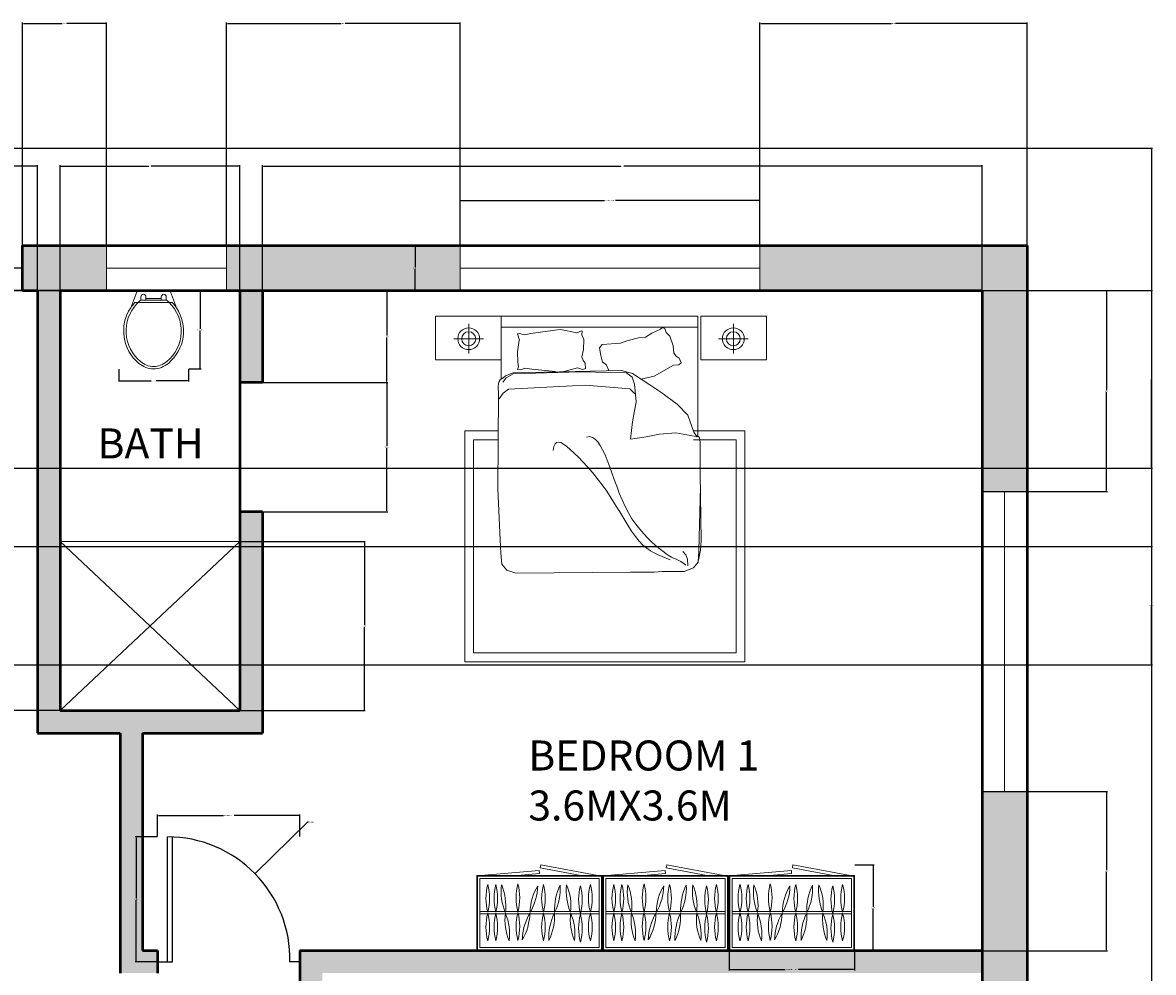
# Model space of a CAD drawing. Units: inches. Extents: x 3 to 380, y -485 to 60.
# Tile 8 of 8: x 154 to 380, y -130 to 60. Entities that reach past the tile are written whole.
import ezdxf

# ---------------------------------------------------------------- set-up
doc = ezdxf.new("R2010")
doc.units = ezdxf.units.IN
doc.header["$MEASUREMENT"] = 0
for name, color, linetype, lineweight in [('A-ANNO-DIMS', 2, 'Continuous', 18), ('A-AREA-IDEN', 7, 'Continuous', 25), ('A-DOOR', 3, 'Continuous', 25), ('A-FLOR-FIXT', 9, 'Continuous', 18), ('A-FURN', 8, 'Continuous', 18), ('A-GLAZ', 4, 'Continuous', 18), ('A-WALL', 7, 'Continuous', 50), ('A-WALL-PATT', 252, 'Continuous', 13)]:
    doc.layers.add(name, color=color, linetype=linetype, lineweight=lineweight)
doc.styles.get("Standard").update_dxf_attribs({"font": 'arial.ttf'})
doc.dimstyles.get("Standard").update_dxf_attribs({"dimtxt": 0.18, "dimasz": 0.18, "dimexe": 0.18, "dimexo": 0.0625, "dimgap": 0.09, "dimtad": 0, "dimtih": 1, "dimtoh": 1, "dimdec": 0, "dimzin": 0, "dimdsep": 46, "dimlunit": 3, "dimtxsty": 'Standard', "dimcen": 0.09, "dimadec": 0, "dimazin": 0, "dimtfac": 1, "dimtdec": 0, "dimtofl": 0, "dimtmove": 0, "dimatfit": 3, "dimfxl": 1, "dimtolj": 1, "dimtzin": 0, "dimarcsym": 0})

# ---------------------------------------------------------------- blocks, each defined once
blk = doc.blocks.new('BED-DOUBLE-WITH-NIGHTSTANDS')
for p, q in [((13.15, 56.48), (13.15, 69.11)), ((6.62, 67.56), (6.62, 61.62)), ((25.02, 66.47), (23.83, 66.33)), ((28.24, 65.8), (25.02, 66.47)), ((29.23, 66.16), (28.24, 65.8)), ((29.33, 66.13), (29.23, 66.16)), ((29.33, 66.13), (29.25, 65.4)), ((29.33, 66.13), (29.25, 65.4)), ((42.02, 64.91), (43.24, 65.73)), ((42.02, 64.91), (43.24, 65.73)), ((43.24, 65.73), (44.98, 66.53)), ((46.15, 65.85), (46.84, 65.09)), ((59.58, 67.56), (59.58, 61.62)), ((3.65, 64.59), (9.59, 64.59)), ((16.76, 64.3), (16.42, 65.57)), ((29.25, 65.4), (29.65, 64.45)), ((29.65, 64.45), (29.63, 62.44)), ((33.33, 63.47), (37.02, 63.69)), ((37.02, 63.69), (38.27, 64.16)), ((38.27, 64.16), (40.63, 64.79)), ((40.63, 64.79), (42.02, 64.91)), ((46.84, 65.09), (47.51, 63.2)), ((62.55, 64.59), (56.61, 64.59)), ((29.63, 62.44), (29.27, 60.96)), ((47.51, 63.2), (47.67, 61.68)), ((47.67, 61.68), (48.15, 61.09)), ((29.27, 60.96), (29.52, 60.24)), ((29.52, 60.24), (29.96, 59.68)), ((29.96, 59.68), (30.03, 58.63)), ((47.6, 59.3), (43.73, 57.13)), ((48.66, 59.34), (47.6, 59.3)), ((48.15, 61.09), (48.75, 60.71)), ((49.17, 59.74), (48.66, 59.34)), ((48.75, 60.71), (49.17, 59.74)), ((28.4, 58.75), (25.21, 57.93)), ((29.41, 58.43), (28.4, 58.75)), ((30.03, 58.63), (29.41, 58.43)), ((12.59, 55.61), (12.54, 55)), ((12.54, 55), (12.56, 53.58)), ((12.56, 53.58), (12.48, 34.55)), ((52.39, 45), (52.46, 45.03)), ((52.97, 37.68), (52.91, 43.85)), ((53.11, 24.16), (52.97, 37.68)), ((12.48, 34.55), (12.89, 24.35)), ((53.02, 35.03), (52.75, 24.82)), ((12.89, 24.35), (13.03, 21.68)), ((52.75, 24.82), (52.69, 22.14)), ((53, 22.29), (53.11, 24.16)), ((13.03, 21.68), (13.27, 19.48)), ((50.1, 21.39), (49.46, 22.06)), ((50.39, 20.5), (50.1, 21.39)), ((50.45, 19.2), (50.39, 20.5)), ((52.69, 22.14), (52.52, 19.94)), ((52.63, 20.34), (53, 22.29)), ((13.27, 19.48), (14.23, 18.32)), ((14.23, 18.32), (16.09, 17.69)), ((51.59, 18.75), (49.75, 18.06)), ((52.52, 19.94), (51.59, 18.75)), ((39.03, 17.94), (16.09, 17.69)), ((39.03, 17.94), (43.71, 17.94)), ((43.71, 17.94), (45.37, 18.06)), ((45.37, 18.06), (49.75, 18.06))]:
    blk.add_line(p, q)
for points in [[(0, 60.38), (13.1, 60.38), (13.1, 69.11), (0, 69.11)], [(66.2, 60.38), (53.1, 60.38), (53.1, 69.11), (66.2, 69.11)]]:
    blk.add_lwpolyline(points, close=True)
for points in [[(13.15, 69.11), (52.45, 69.11), (52.45, 45.06)], [(52.45, 66.93), (13.15, 66.93)], [(23.83, 66.33), (19.08, 65.62), (17.7, 65.39), (16.88, 65.65), (16.42, 65.57)], [(46.15, 65.85), (45.9, 66.66), (45.38, 66.82), (44.98, 66.53)], [(24.02, 58.01), (19.24, 58.51), (17.85, 58.68), (17.04, 58.38), (16.37, 58.47), (16.56, 59), (16.45, 59.9), (16.42, 62), (16.71, 64.3)], [(33.33, 63.47), (32.82, 62.74), (33.06, 61.23), (33.43, 59.89), (34.16, 59.47), (34.58, 58.37), (34.59, 58.17)], [(12.61, 55.65), (12.74, 56.06), (12.92, 56.37), (13.15, 56.48), (13.4, 56.7), (13.44, 56.72)], [(52.45, 44.97), (48.05, 45.75), (44.8, 45.5), (42.14, 44.97), (38.99, 44.52), (39.41, 47.96), (40.12, 51.96), (39.81, 55.5), (39.35, 56.93), (38.2, 57.74), (28.88, 58), (15.49, 57.6), (14.12, 56.79), (13.54, 55.99), (13.47, 55.91)], [(13.48, 56.71), (14.02, 57.18), (15.49, 57.8), (37.2, 58.22), (39.38, 57.66), (42.87, 55.35), (45.06, 53.9), (48.36, 51.48), (50.46, 49.34), (51.7, 45.9), (52.31, 45)], [(43.73, 57.13), (41.15, 56.49)], [(39.86, 53.54), (38.87, 54.55), (30.01, 55.3), (27.42, 55.15), (14.59, 54.51), (13.51, 53.69), (12.69, 52.6)], [(51.61, 46.15), (61.88, 46.15), (61.88, 0), (5.85, 0), (5.85, 46.15), (12.53, 46.15)], [(51.61, 44.4), (60.14, 44.4), (60.14, 1.75), (7.59, 1.75), (7.59, 44.4), (12.53, 44.4)], [(46.96, 20.37), (46.12, 20.73), (45.31, 21.07), (44.52, 21.41), (43.75, 21.77), (42.99, 22.2), (42.24, 22.71), (41.49, 23.33), (40.74, 24.1), (39.99, 25.04), (39.23, 26.12), (38.46, 27.32), (37.67, 28.61), (36.87, 29.96), (36.03, 31.34), (35.16, 32.73), (34.26, 34.09), (33.32, 35.4), (32.36, 36.66), (31.39, 37.84), (30.42, 38.95), (29.48, 39.98), (28.57, 40.91), (27.72, 41.73), (26.93, 42.45), (26.23, 43.05), (25.61, 43.51), (25.06, 43.81), (24.6, 43.93), (24.22, 43.85), (23.91, 43.56), (23.68, 43.04), (23.52, 42.25)], [(50.06, 19.34), (49.7, 19.62), (49.37, 19.84), (49.06, 20.03), (48.78, 20.19), (48.52, 20.33), (48.27, 20.44), (48.02, 20.55), (47.76, 20.67), (47.5, 20.79), (47.21, 20.93), (46.9, 21.1), (46.56, 21.31), (46.16, 21.57), (45.71, 21.89), (45.2, 22.29), (44.61, 22.76), (43.95, 23.32), (43.23, 23.98), (42.45, 24.72), (41.66, 25.56), (40.85, 26.48), (40.05, 27.49), (39.29, 28.58), (38.57, 29.76), (37.91, 31.03), (37.31, 32.35), (36.75, 33.71), (36.24, 35.08), (35.75, 36.45), (35.28, 37.79), (34.82, 39.08), (34.36, 40.29), (33.9, 41.4), (33.43, 42.39), (32.94, 43.25), (32.44, 43.96), (31.91, 44.5), (31.37, 44.86), (30.8, 45.01), (30.2, 44.94)], [(52.91, 43.91), (52.84, 44.76), (52.6, 45.01), (52.45, 45.06)]]:
    blk.add_lwpolyline(points)
for centre, radius in [((6.62, 64.59), 2.18), ((6.62, 64.59), 1.4), ((59.58, 64.59), 2.18), ((59.58, 64.59), 1.4)]:
    blk.add_circle(centre, radius)
blk = doc.blocks.new('WC-PLAN')
for p, q in [((2.25, 13.31), (2.91, 13.31)), ((2.91, 13.31), (5.99, 13.31)), ((9.08, 13.31), (5.99, 13.31)), ((9.08, 13.31), (9.73, 13.31))]:
    blk.add_line(p, q)
for points in [[(5.99, 15.68), (3, 15.68, 0.31031), (2.63, 15.43), (1.4, 12.23, 0.209071)], [(3.45, 13.78, 0.022712), (2.91, 13.31, 0.162618)], [(3.45, 13.78), (3.45, 14.44, -1), (4.45, 14.44), (4.45, 14.1)], [(5.99, 13.78), (3.45, 13.78, 0.022712)], [(5.99, 15.68), (8.98, 15.68, -0.31031), (9.35, 15.43), (10.58, 12.23, -0.209071)], [(5.99, 13.78), (8.53, 13.78, -0.476108)], [(8.53, 13.78), (8.53, 14.44, 1), (7.53, 14.44), (7.53, 14.1)], [(8.53, 13.78, -0.022712), (9.08, 13.31, -0.162618)], [(1.4, 12.23, 0.383919), (3.04, 1.13, 0.163732), (5.99, 0, 0.359733)], [(2.59, 12.99, 0.431639), (3.34, 1.49, 0.162618), (5.99, 0.47, 0.470877)], [(2.25, 13.31, 0.040937), (1.4, 12.23, 0.163732)], [(2.91, 13.31, 0.014165), (2.59, 12.99, 0.162618)], [(9.08, 13.31, -0.448546), (8.64, 1.49, -0.162618), (5.99, 0.47, -0.470877)], [(10.58, 12.23, -0.383919), (8.94, 1.13, -0.163732), (5.99, 0, -0.359733)], [(9.73, 13.31, -0.040937), (10.58, 12.23, -0.163732)]]:
    blk.add_lwpolyline(points, format="xyb")
for points in [[(7.53, 14.1), (4.45, 14.1)], [(4.45, 14.1), (4.45, 13.78)], [(7.53, 14.1), (7.53, 13.78)]]:
    blk.add_lwpolyline(points)
blk = doc.blocks.new('WARDROBE-MODULE')
for p, q in [((0.61, 7.83), (24.49, 7.83)), ((0.61, 7.39), (24.49, 7.39))]:
    blk.add_line(p, q)
for points in [[(0.79, 15.06), (12.48, 16.03), (12.53, 15.42), (8.15, 15.06)], [(24.21, 15.06), (12.8, 17.14), (12.69, 16.54), (20.81, 15.06)]]:
    blk.add_lwpolyline(points)
for points in [[(0, 0), (25.1, 0), (25.1, 15.06), (0, 15.06)], [(0.14, 0.14), (24.96, 0.14), (24.96, 14.92), (0.14, 14.92)], [(0.61, 0.61), (24.49, 0.61), (24.49, 14.45), (0.61, 14.45)]]:
    blk.add_lwpolyline(points, close=True)
for centre, start, end in [((12.71, 10.45), 165.1905, 194.8095), ((-8.32, 10.45), 345.1905, 14.8095), ((14.34, 10.45), 165.1905, 194.8095), ((-6.7, 10.45), 345.1905, 14.8095), ((15.77, 11.77), 172.7904, 202.4093), ((-5.07, 8.99), 352.7904, 22.4093), ((18.76, 10.57), 165.1905, 194.8095), ((-2.27, 10.57), 345.1905, 14.8095), ((1.32, 13.21), 329.2346, 358.8535), ((21.55, 7.43), 149.2346, 178.8535), ((23.87, 10.45), 165.1905, 194.8095), ((2.84, 10.45), 345.1905, 14.8095), ((26.45, 8.28), 153.6481, 183.267), ((5.84, 12.49), 333.6481, 3.267), ((28.79, 11.91), 173.3262, 202.9452), ((7.97, 8.93), 353.3262, 22.9452), ((31.27, 10.2), 165.1905, 194.8095), ((10.24, 10.2), 345.1905, 14.8095), ((33.25, 10.45), 165.1905, 194.8095), ((12.22, 10.45), 345.1905, 14.8095), ((12.71, 4.73), 165.1905, 194.8095), ((-8.32, 4.73), 345.1905, 14.8095), ((14.34, 4.73), 165.1905, 194.8095), ((-6.7, 4.73), 345.1905, 14.8095), ((16.53, 6.1), 172.7904, 202.4093), ((-4.32, 3.32), 352.7904, 22.4093), ((18.76, 4.84), 165.1905, 194.8095), ((-2.27, 4.84), 345.1905, 14.8095), ((19.98, 1.92), 149.2346, 178.8535), ((-0.25, 7.71), 329.2346, 358.8535), ((23.87, 4.73), 165.1905, 194.8095), ((2.84, 4.73), 345.1905, 14.8095), ((25.3, 2.68), 153.6481, 183.267), ((4.69, 6.89), 333.6481, 3.267), ((29.6, 6.25), 173.3262, 202.9452), ((8.78, 3.27), 353.3262, 22.9452), ((31.27, 4.48), 165.1905, 194.8095), ((10.24, 4.48), 345.1905, 14.8095), ((33.25, 4.73), 165.1905, 194.8095), ((12.22, 4.73), 345.1905, 14.8095)]:
    blk.add_arc(centre, 10.88, start, end)
blk = doc.blocks.new('WIN-60X9')
for p, q in [((60, 9), (0, 9)), ((0, 9), (0, 0)), ((60, 0), (60, 9)), ((0, 4.5), (60, 4.5)), ((0, 0), (60, 0))]:
    blk.add_line(p, q)
blk = doc.blocks.new('WIN-24X9')
for p, q in [((0, 24), (0, 0)), ((9, 24), (0, 24)), ((4.5, 24), (4.5, 0)), ((9, 0), (9, 24)), ((0, 0), (9, 0))]:
    blk.add_line(p, q)
blk = doc.blocks.new('DOOR-SWING-24')
for p, q in [((25, 0), (25, 24)), ((26, 0), (26, 24)), ((2, 0), (0, 0)), ((25, 0), (26, 0)), ((28, 0), (26, 0))]:
    blk.add_line(p, q)
blk.add_arc((26, 0), 24, 90, 180)
blk = doc.blocks.new('DOOR-SWING-25')
for p, q in [((2, 0), (2, 25)), ((3, 0), (3, 25)), ((0, 0), (2, 0)), ((2, 0), (3, 0)), ((28.5, 0), (26.5, 0))]:
    blk.add_line(p, q)
blk.add_arc((2, 0.5), 24.5, 358.8425, 90)
blk = doc.blocks.new('*D17')
at = {"layer": 'A-ANNO-DIMS', "color": 0, "lineweight": -2, "transparency": 16777216}
for p, q in [((241.37, 15.23), (241.37, 24.34)), ((241.55, 24.16), (270.26, 24.16)), ((301.19, 24.16), (272.49, 24.16)), ((301.37, 15.23), (301.37, 24.34))]:
    blk.add_line(p, q, dxfattribs=at)
at = {"layer": 'A-ANNO-DIMS', "color": 0, "transparency": 16777216}
for points in [[(241.55, 24.19), (241.55, 24.13), (241.37, 24.16)], [(301.19, 24.19), (301.19, 24.13), (301.37, 24.16)]]:
    blk.add_solid(points, dxfattribs=at)
at = {"layer": 'Defpoints', "color": 0, "transparency": 16777216}
for p in [(301.37, 24.16), (241.37, 15.16), (301.37, 15.16)]:
    blk.add_point(p, dxfattribs=at)
at = {"layer": 'A-ANNO-DIMS', "color": 0, "transparency": 16777216, "insert": (271.37, 24.16), "char_height": 0.18, "attachment_point": 5}
blk.add_mtext('\\A1;WINDOW 60 TYP.', dxfattribs=at)
blk = doc.blocks.new('*D18')
at = {"layer": 'A-ANNO-DIMS', "color": 0, "lineweight": -2, "transparency": 16777216}
for p, q in [((241.31, 15.16), (232.19, 15.16)), ((232.37, 14.98), (232.37, 10.85)), ((232.37, 6.34), (232.37, 10.48)), ((241.31, 6.16), (232.19, 6.16))]:
    blk.add_line(p, q, dxfattribs=at)
at = {"layer": 'A-ANNO-DIMS', "color": 0, "transparency": 16777216}
for points in [[(232.34, 14.98), (232.4, 14.98), (232.37, 15.16)], [(232.34, 6.34), (232.4, 6.34), (232.37, 6.16)]]:
    blk.add_solid(points, dxfattribs=at)
at = {"layer": 'Defpoints', "color": 0, "transparency": 16777216}
for p in [(232.37, 15.16), (241.37, 15.16), (241.37, 6.16)]:
    blk.add_point(p, dxfattribs=at)
at = {"layer": 'A-ANNO-DIMS', "color": 0, "transparency": 16777216, "insert": (232.37, 10.66), "char_height": 0.18, "attachment_point": 5}
blk.add_mtext('\\A1;9 TYP.', dxfattribs=at)
blk = doc.blocks.new('*D25')
at = {"layer": 'A-ANNO-DIMS', "color": 0, "lineweight": -2, "transparency": 16777216}
for p, q in [((180.84, -103.02), (180.84, -98.63)), ((181.02, -98.81), (194.04, -98.81)), ((209.16, -98.81), (196.14, -98.81)), ((209.34, -103.02), (209.34, -98.63))]:
    blk.add_line(p, q, dxfattribs=at)
at = {"layer": 'A-ANNO-DIMS', "color": 0, "transparency": 16777216}
for points in [[(181.02, -98.78), (181.02, -98.84), (180.84, -98.81)], [(209.16, -98.78), (209.16, -98.84), (209.34, -98.81)]]:
    blk.add_solid(points, dxfattribs=at)
at = {"layer": 'Defpoints', "color": 0, "transparency": 16777216}
for p in [(209.34, -98.81), (180.84, -103.09), (209.34, -103.09)]:
    blk.add_point(p, dxfattribs=at)
at = {"layer": 'A-ANNO-DIMS', "color": 0, "transparency": 16777216, "insert": (195.09, -98.81), "char_height": 0.18, "attachment_point": 5}
blk.add_mtext('\\A1;DOOR B 29 TYP.', dxfattribs=at)
blk = doc.blocks.new('*D26')
at = {"layer": 'A-ANNO-DIMS', "color": 0, "lineweight": -2, "transparency": 16777216}
for p, q in [((180.78, -103.09), (176.39, -103.09)), ((176.57, -103.27), (176.57, -115.4)), ((176.57, -127.91), (176.57, -115.77)), ((180.78, -128.09), (176.39, -128.09))]:
    blk.add_line(p, q, dxfattribs=at)
at = {"layer": 'A-ANNO-DIMS', "color": 0, "transparency": 16777216}
for points in [[(176.54, -103.27), (176.6, -103.27), (176.57, -103.09)], [(176.54, -127.91), (176.6, -127.91), (176.57, -128.09)]]:
    blk.add_solid(points, dxfattribs=at)
at = {"layer": 'Defpoints', "color": 0, "transparency": 16777216}
for p in [(176.57, -103.09), (180.84, -103.09), (180.84, -128.09)]:
    blk.add_point(p, dxfattribs=at)
at = {"layer": 'A-ANNO-DIMS', "color": 0, "transparency": 16777216, "insert": (176.57, -115.59), "char_height": 0.18, "attachment_point": 5}
blk.add_mtext('\\A1;25 TYP.', dxfattribs=at)
blk = doc.blocks.new('*D29')
at = {"layer": 'A-ANNO-DIMS', "color": 0, "lineweight": -2, "transparency": 16777216}
for p, q in [((295.2, -125.9), (295.2, -129.78)), ((320.3, -125.9), (320.3, -129.78)), ((295.38, -129.6), (306.44, -129.6)), ((320.12, -129.6), (309.06, -129.6))]:
    blk.add_line(p, q, dxfattribs=at)
at = {"layer": 'A-ANNO-DIMS', "color": 0, "transparency": 16777216}
for points in [[(295.38, -129.57), (295.38, -129.63), (295.2, -129.6)], [(320.12, -129.57), (320.12, -129.63), (320.3, -129.6)]]:
    blk.add_solid(points, dxfattribs=at)
at = {"layer": 'Defpoints', "color": 0, "transparency": 16777216}
for p in [(295.2, -125.84), (320.3, -125.84), (320.3, -129.6)]:
    blk.add_point(p, dxfattribs=at)
at = {"layer": 'A-ANNO-DIMS', "color": 0, "transparency": 16777216, "insert": (307.75, -129.6), "char_height": 0.18, "attachment_point": 5}
blk.add_mtext('\\A1;WARDROBE 25 TYP.', dxfattribs=at)
blk = doc.blocks.new('*D30')
at = {"layer": 'A-ANNO-DIMS', "color": 0, "lineweight": -2, "transparency": 16777216}
for p, q in [((320.36, -108.7), (324.24, -108.7)), ((324.06, -108.88), (324.06, -117.09)), ((324.06, -125.66), (324.06, -117.45)), ((320.36, -125.84), (324.24, -125.84))]:
    blk.add_line(p, q, dxfattribs=at)
at = {"layer": 'A-ANNO-DIMS', "color": 0, "transparency": 16777216}
for points in [[(324.03, -108.88), (324.09, -108.88), (324.06, -108.7)], [(324.03, -125.66), (324.09, -125.66), (324.06, -125.84)]]:
    blk.add_solid(points, dxfattribs=at)
at = {"layer": 'Defpoints', "color": 0, "transparency": 16777216}
for p in [(320.3, -108.7), (324.06, -108.7), (320.3, -125.84)]:
    blk.add_point(p, dxfattribs=at)
at = {"layer": 'A-ANNO-DIMS', "color": 0, "transparency": 16777216, "insert": (324.06, -117.27), "char_height": 0.18, "attachment_point": 5}
blk.add_mtext('\\A1;17 TYP.', dxfattribs=at)
blk = doc.blocks.new('*D33')
at = {"layer": 'A-ANNO-DIMS', "color": 0, "lineweight": -2, "transparency": 16777216}
for p, q in [((187.08, 6.16), (189.55, 6.16)), ((189.37, 5.98), (189.37, -1.49)), ((189.37, -9.34), (189.37, -1.86)), ((187.08, -9.52), (189.55, -9.52))]:
    blk.add_line(p, q, dxfattribs=at)
at = {"layer": 'A-ANNO-DIMS', "color": 0, "transparency": 16777216}
for points in [[(189.34, 5.98), (189.4, 5.98), (189.37, 6.16)], [(189.34, -9.34), (189.4, -9.34), (189.37, -9.52)]]:
    blk.add_solid(points, dxfattribs=at)
at = {"layer": 'Defpoints', "color": 0, "transparency": 16777216}
for p in [(187.02, 6.16), (189.37, 6.16), (187.02, -9.52)]:
    blk.add_point(p, dxfattribs=at)
at = {"layer": 'A-ANNO-DIMS', "color": 0, "transparency": 16777216, "insert": (189.37, -1.68), "char_height": 0.18, "attachment_point": 5}
blk.add_mtext('\\A1;WC 16 TYP.', dxfattribs=at)
blk = doc.blocks.new('*D34')
at = {"layer": 'A-ANNO-DIMS', "color": 0, "lineweight": -2, "transparency": 16777216}
for p, q in [((173.09, -9.58), (173.09, -12.05)), ((187.02, -9.58), (187.02, -12.05)), ((173.27, -11.87), (179.54, -11.87)), ((186.84, -11.87), (180.58, -11.87))]:
    blk.add_line(p, q, dxfattribs=at)
at = {"layer": 'A-ANNO-DIMS', "color": 0, "transparency": 16777216}
for points in [[(173.27, -11.84), (173.27, -11.9), (173.09, -11.87)], [(186.84, -11.84), (186.84, -11.9), (187.02, -11.87)]]:
    blk.add_solid(points, dxfattribs=at)
at = {"layer": 'Defpoints', "color": 0, "transparency": 16777216}
for p in [(173.09, -9.52), (187.02, -9.52), (187.02, -11.87)]:
    blk.add_point(p, dxfattribs=at)
at = {"layer": 'A-ANNO-DIMS', "color": 0, "transparency": 16777216, "insert": (180.06, -11.87), "char_height": 0.18, "attachment_point": 5}
blk.add_mtext('\\A1;14 TYP.', dxfattribs=at)
blk = doc.blocks.new('*D51')
at = {"layer": 'A-ANNO-DIMS', "color": 0, "lineweight": -2, "transparency": 16777216}
for p, q in [((151.9, 34.66), (379.92, 34.66)), ((379.74, 34.48), (379.74, -212.65)), ((379.74, -460.16), (379.74, -213.02)), ((354.9, -460.34), (379.92, -460.34))]:
    blk.add_line(p, q, dxfattribs=at)
at = {"layer": 'A-ANNO-DIMS', "color": 0, "transparency": 16777216}
for points in [[(379.71, 34.48), (379.77, 34.48), (379.74, 34.66)], [(379.71, -460.16), (379.77, -460.16), (379.74, -460.34)]]:
    blk.add_solid(points, dxfattribs=at)
at = {"layer": 'Defpoints', "color": 0, "transparency": 16777216}
for p in [(151.84, 34.66), (354.84, -460.34), (379.74, -460.34)]:
    blk.add_point(p, dxfattribs=at)
at = {"layer": 'A-ANNO-DIMS', "color": 0, "transparency": 16777216, "insert": (379.74, -212.84), "char_height": 0.18, "attachment_point": 5}
blk.add_mtext('\\A1;495', dxfattribs=at)
blk = doc.blocks.new('*D59')
at = {"layer": 'A-ANNO-DIMS', "color": 0, "lineweight": -2, "transparency": 16777216}
for p, q in [((153.84, 15.23), (153.84, 59.74)), ((154.02, 59.56), (161.78, 59.56)), ((170.46, 59.56), (162.69, 59.56)), ((170.64, 15.23), (170.64, 59.74))]:
    blk.add_line(p, q, dxfattribs=at)
at = {"layer": 'A-ANNO-DIMS', "color": 0, "transparency": 16777216}
for points in [[(154.02, 59.59), (154.02, 59.53), (153.84, 59.56)], [(170.46, 59.59), (170.46, 59.53), (170.64, 59.56)]]:
    blk.add_solid(points, dxfattribs=at)
at = {"layer": 'Defpoints', "color": 0, "transparency": 16777216}
for p in [(170.64, 59.56), (153.84, 15.16), (170.64, 15.16)]:
    blk.add_point(p, dxfattribs=at)
at = {"layer": 'A-ANNO-DIMS', "color": 0, "transparency": 16777216, "insert": (162.24, 59.56), "char_height": 0.18, "attachment_point": 5}
blk.add_mtext('\\A1;16.795', dxfattribs=at)
blk = doc.blocks.new('*D60')
at = {"layer": 'A-ANNO-DIMS', "color": 0, "lineweight": -2, "transparency": 16777216}
for p, q in [((194.64, 15.23), (194.64, 59.74)), ((194.82, 59.56), (217.61, 59.56)), ((241.19, 59.56), (218.4, 59.56)), ((241.37, 15.23), (241.37, 59.74))]:
    blk.add_line(p, q, dxfattribs=at)
at = {"layer": 'A-ANNO-DIMS', "color": 0, "transparency": 16777216}
for points in [[(194.82, 59.59), (194.82, 59.53), (194.64, 59.56)], [(241.19, 59.59), (241.19, 59.53), (241.37, 59.56)]]:
    blk.add_solid(points, dxfattribs=at)
at = {"layer": 'Defpoints', "color": 0, "transparency": 16777216}
for p in [(241.37, 59.56), (194.64, 15.16), (241.37, 15.16)]:
    blk.add_point(p, dxfattribs=at)
at = {"layer": 'A-ANNO-DIMS', "color": 0, "transparency": 16777216, "insert": (218, 59.56), "char_height": 0.18, "attachment_point": 5}
blk.add_mtext('\\A1;46.74', dxfattribs=at)
blk = doc.blocks.new('*D61')
at = {"layer": 'A-ANNO-DIMS', "color": 0, "lineweight": -2, "transparency": 16777216}
for p, q in [((301.37, 15.23), (301.37, 59.74)), ((301.55, 59.56), (327.71, 59.56)), ((354.66, 59.56), (328.5, 59.56)), ((354.84, 15.23), (354.84, 59.74))]:
    blk.add_line(p, q, dxfattribs=at)
at = {"layer": 'A-ANNO-DIMS', "color": 0, "transparency": 16777216}
for points in [[(301.55, 59.59), (301.55, 59.53), (301.37, 59.56)], [(354.66, 59.59), (354.66, 59.53), (354.84, 59.56)]]:
    blk.add_solid(points, dxfattribs=at)
at = {"layer": 'Defpoints', "color": 0, "transparency": 16777216}
for p in [(354.84, 59.56), (301.37, 15.16), (354.84, 15.16)]:
    blk.add_point(p, dxfattribs=at)
at = {"layer": 'A-ANNO-DIMS', "color": 0, "transparency": 16777216, "insert": (328.11, 59.56), "char_height": 0.18, "attachment_point": 5}
blk.add_mtext('\\A1;53.47', dxfattribs=at)
blk = doc.blocks.new('*D62')
at = {"layer": 'A-ANNO-DIMS', "color": 0, "lineweight": -2, "transparency": 16777216}
for p, q in [((345.9, 6.16), (370.92, 6.16)), ((370.74, 5.98), (370.74, -13.75)), ((370.74, -33.85), (370.74, -14.12)), ((345.9, -34.03), (370.92, -34.03))]:
    blk.add_line(p, q, dxfattribs=at)
at = {"layer": 'A-ANNO-DIMS', "color": 0, "transparency": 16777216}
for points in [[(370.71, 5.98), (370.77, 5.98), (370.74, 6.16)], [(370.71, -33.85), (370.77, -33.85), (370.74, -34.03)]]:
    blk.add_solid(points, dxfattribs=at)
at = {"layer": 'Defpoints', "color": 0, "transparency": 16777216}
for p in [(345.84, 6.16), (345.84, -34.03), (370.74, -34.03)]:
    blk.add_point(p, dxfattribs=at)
at = {"layer": 'A-ANNO-DIMS', "color": 0, "transparency": 16777216, "insert": (370.74, -13.93), "char_height": 0.18, "attachment_point": 5}
blk.add_mtext('\\A1;40.2', dxfattribs=at)
blk = doc.blocks.new('*D63')
at = {"layer": 'A-ANNO-DIMS', "color": 0, "lineweight": -2, "transparency": 16777216}
for p, q in [((345.9, -94.03), (370.92, -94.03)), ((370.74, -94.21), (370.74, -109.75)), ((370.74, -125.66), (370.74, -110.12)), ((345.9, -125.84), (370.92, -125.84))]:
    blk.add_line(p, q, dxfattribs=at)
at = {"layer": 'A-ANNO-DIMS', "color": 0, "transparency": 16777216}
for points in [[(370.71, -94.21), (370.77, -94.21), (370.74, -94.03)], [(370.71, -125.66), (370.77, -125.66), (370.74, -125.84)]]:
    blk.add_solid(points, dxfattribs=at)
at = {"layer": 'Defpoints', "color": 0, "transparency": 16777216}
for p in [(345.84, -94.03), (345.84, -125.84), (370.74, -125.84)]:
    blk.add_point(p, dxfattribs=at)
at = {"layer": 'A-ANNO-DIMS', "color": 0, "transparency": 16777216, "insert": (370.74, -109.93), "char_height": 0.18, "attachment_point": 5}
blk.add_mtext('\\A1;31.8', dxfattribs=at)
blk = doc.blocks.new('*D70')
at = {"layer": 'A-ANNO-DIMS', "color": 0, "lineweight": -2, "transparency": 16777216}
for p, q in [((36.84, 6.23), (36.84, 31.24)), ((37.02, 31.06), (96.56, 31.06)), ((156.66, 31.06), (97.12, 31.06)), ((156.84, 6.23), (156.84, 31.24))]:
    blk.add_line(p, q, dxfattribs=at)
at = {"layer": 'A-ANNO-DIMS', "color": 0, "transparency": 16777216}
for points in [[(37.02, 31.09), (37.02, 31.03), (36.84, 31.06)], [(156.66, 31.09), (156.66, 31.03), (156.84, 31.06)]]:
    blk.add_solid(points, dxfattribs=at)
at = {"layer": 'Defpoints', "color": 0, "transparency": 16777216}
for p in [(156.84, 31.06), (36.84, 6.16), (156.84, 6.16)]:
    blk.add_point(p, dxfattribs=at)
at = {"layer": 'A-ANNO-DIMS', "color": 0, "transparency": 16777216, "insert": (96.84, 31.06), "char_height": 0.18, "attachment_point": 5}
blk.add_mtext('\\A1;120', dxfattribs=at)
blk = doc.blocks.new('*D71')
at = {"layer": 'A-ANNO-DIMS', "color": 0, "lineweight": -2, "transparency": 16777216}
for p, q in [((161.28, 6.16), (136.26, 6.16)), ((136.44, 5.98), (136.44, -35.65)), ((136.44, -77.66), (136.44, -36.02)), ((161.28, -77.84), (136.26, -77.84))]:
    blk.add_line(p, q, dxfattribs=at)
at = {"layer": 'A-ANNO-DIMS', "color": 0, "transparency": 16777216}
for points in [[(136.41, 5.98), (136.47, 5.98), (136.44, 6.16)], [(136.41, -77.66), (136.47, -77.66), (136.44, -77.84)]]:
    blk.add_solid(points, dxfattribs=at)
at = {"layer": 'Defpoints', "color": 0, "transparency": 16777216}
for p in [(136.44, 6.16), (161.34, 6.16), (161.34, -77.84)]:
    blk.add_point(p, dxfattribs=at)
at = {"layer": 'A-ANNO-DIMS', "color": 0, "transparency": 16777216, "insert": (136.44, -35.84), "char_height": 0.18, "attachment_point": 5}
blk.add_mtext('\\A1;84', dxfattribs=at)
blk = doc.blocks.new('*D72')
at = {"layer": 'A-ANNO-DIMS', "color": 0, "lineweight": -2, "transparency": 16777216}
for p, q in [((161.34, 6.23), (161.34, 31.24)), ((161.52, 31.06), (179.12, 31.06)), ((197.16, 31.06), (179.56, 31.06)), ((197.34, 6.23), (197.34, 31.24))]:
    blk.add_line(p, q, dxfattribs=at)
at = {"layer": 'A-ANNO-DIMS', "color": 0, "transparency": 16777216}
for points in [[(161.52, 31.09), (161.52, 31.03), (161.34, 31.06)], [(197.16, 31.09), (197.16, 31.03), (197.34, 31.06)]]:
    blk.add_solid(points, dxfattribs=at)
at = {"layer": 'Defpoints', "color": 0, "transparency": 16777216}
for p in [(197.34, 31.06), (161.34, 6.16), (197.34, 6.16)]:
    blk.add_point(p, dxfattribs=at)
at = {"layer": 'A-ANNO-DIMS', "color": 0, "transparency": 16777216, "insert": (179.34, 31.06), "char_height": 0.18, "attachment_point": 5}
blk.add_mtext('\\A1;36', dxfattribs=at)
blk = doc.blocks.new('*D73')
at = {"layer": 'A-ANNO-DIMS', "color": 0, "lineweight": -2, "transparency": 16777216}
for p, q in [((201.84, 6.23), (201.84, 31.24)), ((202.02, 31.06), (273.56, 31.06)), ((345.66, 31.06), (274.12, 31.06)), ((345.84, 6.23), (345.84, 31.24))]:
    blk.add_line(p, q, dxfattribs=at)
at = {"layer": 'A-ANNO-DIMS', "color": 0, "transparency": 16777216}
for points in [[(202.02, 31.09), (202.02, 31.03), (201.84, 31.06)], [(345.66, 31.09), (345.66, 31.03), (345.84, 31.06)]]:
    blk.add_solid(points, dxfattribs=at)
at = {"layer": 'Defpoints', "color": 0, "transparency": 16777216}
for p in [(345.84, 31.06), (201.84, 6.16), (345.84, 6.16)]:
    blk.add_point(p, dxfattribs=at)
at = {"layer": 'A-ANNO-DIMS', "color": 0, "transparency": 16777216, "insert": (273.84, 31.06), "char_height": 0.18, "attachment_point": 5}
blk.add_mtext('\\A1;144', dxfattribs=at)
blk = doc.blocks.new('*D74')
at = {"layer": 'A-ANNO-DIMS', "color": 0, "lineweight": -2, "transparency": 16777216}
for p, q in [((201.9, -12.2), (226.92, -12.2)), ((226.74, -12.38), (226.74, -24.96)), ((226.74, -37.91), (226.74, -25.32)), ((201.9, -38.09), (226.92, -38.09))]:
    blk.add_line(p, q, dxfattribs=at)
at = {"layer": 'A-ANNO-DIMS', "color": 0, "transparency": 16777216}
for points in [[(226.71, -12.38), (226.77, -12.38), (226.74, -12.2)], [(226.71, -37.91), (226.77, -37.91), (226.74, -38.09)]]:
    blk.add_solid(points, dxfattribs=at)
at = {"layer": 'Defpoints', "color": 0, "transparency": 16777216}
for p in [(201.84, -12.2), (201.84, -38.09), (226.74, -38.09)]:
    blk.add_point(p, dxfattribs=at)
at = {"layer": 'A-ANNO-DIMS', "color": 0, "transparency": 16777216, "insert": (226.74, -25.14), "char_height": 0.18, "attachment_point": 5}
blk.add_mtext('\\A1;25.89', dxfattribs=at)
blk = doc.blocks.new('*D75')
at = {"layer": 'A-ANNO-DIMS', "color": 0, "lineweight": -2, "transparency": 16777216}
for p, q in [((201.9, 6.16), (226.92, 6.16)), ((226.74, 5.98), (226.74, -2.83)), ((226.74, -12.02), (226.74, -3.2)), ((201.9, -12.2), (226.92, -12.2))]:
    blk.add_line(p, q, dxfattribs=at)
at = {"layer": 'A-ANNO-DIMS', "color": 0, "transparency": 16777216}
for points in [[(226.71, 5.98), (226.77, 5.98), (226.74, 6.16)], [(226.71, -12.02), (226.77, -12.02), (226.74, -12.2)]]:
    blk.add_solid(points, dxfattribs=at)
at = {"layer": 'Defpoints', "color": 0, "transparency": 16777216}
for p in [(201.84, 6.16), (201.84, -12.2), (226.74, -12.2)]:
    blk.add_point(p, dxfattribs=at)
at = {"layer": 'A-ANNO-DIMS', "color": 0, "transparency": 16777216, "insert": (226.74, -3.02), "char_height": 0.18, "attachment_point": 5}
blk.add_mtext('\\A1;18.362', dxfattribs=at)
blk = doc.blocks.new('*D76')
at = {"layer": 'A-ANNO-DIMS', "color": 0, "lineweight": -2, "transparency": 16777216}
for p, q in [((197.4, -44.03), (222.42, -44.03)), ((222.24, -44.21), (222.24, -60.75)), ((222.24, -77.66), (222.24, -61.12)), ((197.4, -77.84), (222.42, -77.84))]:
    blk.add_line(p, q, dxfattribs=at)
at = {"layer": 'A-ANNO-DIMS', "color": 0, "transparency": 16777216}
for points in [[(222.21, -44.21), (222.27, -44.21), (222.24, -44.03)], [(222.21, -77.66), (222.27, -77.66), (222.24, -77.84)]]:
    blk.add_solid(points, dxfattribs=at)
at = {"layer": 'Defpoints', "color": 0, "transparency": 16777216}
for p in [(197.34, -44.03), (197.34, -77.84), (222.24, -77.84)]:
    blk.add_point(p, dxfattribs=at)
at = {"layer": 'A-ANNO-DIMS', "color": 0, "transparency": 16777216, "insert": (222.24, -60.93), "char_height": 0.18, "attachment_point": 5}
blk.add_mtext('\\A1;33.8', dxfattribs=at)
blk = doc.blocks.new('*D91')
at = {"layer": 'A-ANNO-DIMS', "color": 0, "lineweight": -2, "transparency": 16777216}
for p, q in [((122.68, 6.16), (379.92, 6.16)), ((379.74, 5.98), (379.74, -11.4)), ((379.74, -29.16), (379.74, -11.77)), ((122.68, -29.34), (379.92, -29.34))]:
    blk.add_line(p, q, dxfattribs=at)
at = {"layer": 'A-ANNO-DIMS', "color": 0, "transparency": 16777216}
for points in [[(379.71, 5.98), (379.77, 5.98), (379.74, 6.16)], [(379.71, -29.16), (379.77, -29.16), (379.74, -29.34)]]:
    blk.add_solid(points, dxfattribs=at)
at = {"layer": 'Defpoints', "color": 0, "transparency": 16777216}
for p in [(122.62, 6.16), (122.62, -29.34), (379.74, -29.34)]:
    blk.add_point(p, dxfattribs=at)
at = {"layer": 'A-ANNO-DIMS', "color": 0, "transparency": 16777216, "insert": (379.74, -11.59), "char_height": 0.18, "attachment_point": 5}
blk.add_mtext('\\A1;35.5', dxfattribs=at)
blk = doc.blocks.new('*D96')
at = {"layer": 'A-ANNO-DIMS', "color": 0, "lineweight": -2, "transparency": 16777216}
for p, q in [((60.16, -44.99), (379.92, -44.99)), ((379.74, -45.17), (379.74, -56.64)), ((379.74, -68.49), (379.74, -57.01)), ((60.16, -68.67), (379.92, -68.67))]:
    blk.add_line(p, q, dxfattribs=at)
at = {"layer": 'A-ANNO-DIMS', "color": 0, "transparency": 16777216}
for points in [[(379.71, -45.17), (379.77, -45.17), (379.74, -44.99)], [(379.71, -68.49), (379.77, -68.49), (379.74, -68.67)]]:
    blk.add_solid(points, dxfattribs=at)
at = {"layer": 'Defpoints', "color": 0, "transparency": 16777216}
for p in [(60.09, -44.99), (60.09, -68.67), (379.74, -68.67)]:
    blk.add_point(p, dxfattribs=at)
at = {"layer": 'A-ANNO-DIMS', "color": 0, "transparency": 16777216, "insert": (379.74, -56.83), "char_height": 0.18, "attachment_point": 5}
blk.add_mtext('\\A1;23.683', dxfattribs=at)
blk = doc.blocks.new('*D103')
at = {"layer": 'A-ANNO-DIMS', "color": 0, "lineweight": -2, "transparency": 16777216}
for p, q in [((210.84, -100.15), (200.47, -110.31)), ((211.02, -100.15), (210.84, -100.15)), ((182.75, -127.59), (182.93, -127.59)), ((182.84, -127.68), (182.84, -127.5))]:
    blk.add_line(p, q, dxfattribs=at)
at = {"layer": 'A-ANNO-DIMS', "color": 0, "transparency": 16777216}
blk.add_solid([(200.45, -110.29), (200.49, -110.33), (200.34, -110.44)], dxfattribs=at)
at = {"layer": 'Defpoints', "color": 0, "transparency": 16777216}
for p in [(200.34, -110.44), (182.84, -127.59)]:
    blk.add_point(p, dxfattribs=at)
at = {"layer": 'A-ANNO-DIMS', "color": 0, "transparency": 16777216, "insert": (211.57, -100.15), "char_height": 0.18, "attachment_point": 5}
blk.add_mtext('\\A1;R24.505', dxfattribs=at)

msp = doc.modelspace()

# ---------------------------------------------------------------- hatches: boundary and pattern name
at = {"layer": 'A-WALL-PATT'}
h = msp.add_hatch(color=256, dxfattribs=at)
h.dxf.hatch_style = 1
h.paths.add_polyline_path([(36.8404, 6.1643), (51.3404, 6.1643), (51.3404, 15.1643), (27.8404, 15.1643), (27.8404, -143.6318), (36.8404, -143.6318)])
h.paths.add_polyline_path([(125.8404, 10.6643), (125.8404, 15.1643), (111.3404, 15.1643), (111.3404, 6.1643), (125.8404, 6.1643)])
h.paths.add_polyline_path([(170.6358, 15.1643), (153.8404, 15.1643), (153.8404, 6.1643), (156.8404, 6.1643), (156.8404, -82.3357), (173.3404, -82.3357), (173.3404, -130.3357), (177.8404, -130.3357), (180.8404, -130.3357), (180.8404, -125.8357), (177.8404, -125.8357), (177.8404, -82.3357), (201.8404, -82.3357), (201.8404, -38.0857), (197.3404, -38.0857), (197.3404, -77.8357), (161.3404, -77.8357), (161.3404, 6.1643), (170.6358, 6.1643)])
h.paths.add_polyline_path([(241.3739, 15.1643), (194.6358, 15.1643), (194.6358, 6.1643), (241.3739, 6.1643)])
h.paths.add_polyline_path([(201.8404, 6.1643), (197.3404, 6.1643), (197.3404, -12.1977), (201.8404, -12.1977)], flags=17)
h.paths.add_polyline_path([(354.8404, 15.1643), (301.3739, 15.1643), (301.3739, 6.1643), (345.8404, 6.1643), (345.8404, -34.0336), (354.8404, -34.0336)])
h.paths.add_polyline_path([(354.8404, -94.0336), (345.8404, -94.0336), (345.8404, -159.3738), (354.8404, -159.3738)])
h.paths.add_polyline_path([(345.8404, -125.8357), (209.3404, -125.8357), (209.3404, -205.8357), (211.5904, -205.8357), (213.8404, -205.8357), (213.8404, -130.3357), (345.8404, -130.3357)])
h.paths.add_polyline_path([(36.8404, -203.6318), (27.8404, -203.6318), (27.8404, -270.1269), (36.8404, -270.1269)])
h.paths.add_polyline_path([(36.8404, -330.1269), (27.8404, -330.1269), (27.8404, -362.428), (57.3404, -362.428), (57.3404, -353.428), (36.8404, -353.428)])
h.paths.add_polyline_path([(177.8404, -331.3357), (180.8404, -331.3357), (180.8404, -326.8357), (173.3404, -326.8357), (173.3404, -353.428), (165.8404, -353.428), (165.8404, -362.428), (168.8404, -362.428), (168.8404, -451.3357), (168.8404, -460.3357), (231.8404, -460.3357), (231.8404, -451.3357), (177.8404, -451.3357)])
h.paths.add_polyline_path([(354.8404, -305.1003), (345.8404, -305.1003), (345.8404, -363.2829), (354.8404, -363.2829)])
h.paths.add_polyline_path([(345.8404, -326.8357), (213.8404, -326.8357), (213.8404, -312.8357), (211.5904, -312.8357), (209.3404, -312.8357), (209.3404, -331.3357), (345.8404, -331.3357)])
h.paths.add_polyline_path([(345.8404, -262.3357), (237.8404, -262.3357), (237.8404, -233.8357), (209.3404, -233.8357), (209.3404, -284.8357), (213.8404, -284.8357), (213.8404, -238.3357), (233.3404, -238.3357), (233.3404, -266.8357), (345.8404, -266.8357)])
h.paths.add_polyline_path([(354.8404, -219.3738), (345.8404, -219.3738), (345.8404, -281.1003), (354.8404, -281.1003)])

# ---------------------------------------------------------------- linework, layer by layer
at = {"layer": 'A-FLOR-FIXT'}
for p, q in [((197.3404, -44.0331), (161.3404, -44.0331)), ((161.3404, -44.0331), (197.3404, -77.8357)), ((197.3404, -44.0331), (161.3404, -77.8357))]:
    msp.add_line(p, q, dxfattribs=at)
at = {"layer": 'A-WALL'}
for p, q in [((153.8404, 6.1643), (153.8404, 15.1643)), ((153.8404, 15.1643), (354.8404, 15.1643)), ((354.8404, 15.1643), (354.8404, -460.3357)), ((153.8404, 6.1643), (156.8404, 6.1643)), ((156.8404, 6.1643), (156.8404, -82.3357)), ((161.3404, 6.1643), (161.3404, -77.8357)), ((161.3404, 6.1643), (345.8404, 6.1643)), ((197.3404, 6.1643), (197.3404, -77.8357)), ((201.8404, 6.1643), (201.8404, -12.1977)), ((345.8404, 6.1643), (345.8404, -451.3357)), ((201.8404, -12.1977), (197.3404, -12.1977)), ((201.8404, -38.0857), (197.3404, -38.0857)), ((201.8404, -38.0857), (201.8404, -82.3357)), ((161.3404, -77.8357), (197.3404, -77.8357)), ((156.8404, -82.3357), (173.3404, -82.3357)), ((173.3404, -82.3357), (173.3404, -130.3357)), ((177.8404, -82.3357), (177.8404, -125.8357)), ((177.8404, -82.3357), (201.8404, -82.3357)), ((177.8404, -125.8357), (180.8404, -125.8357)), ((180.8404, -125.8357), (180.8404, -130.3357)), ((209.3404, -125.8357), (345.8404, -125.8357)), ((209.3404, -125.8357), (209.3404, -205.8357))]:
    msp.add_line(p, q, dxfattribs=at)

# ---------------------------------------------------------------- block references
at = {"layer": 'A-DOOR'}
for name, p in [('DOOR-SWING-24', (125.84, 10.664)), ('DOOR-SWING-25', (180.84, -128.086))]:
    msp.add_blockref(name, p, dxfattribs=at)
at = {"layer": 'A-FLOR-FIXT'}
msp.add_blockref('WC-PLAN', (174.066, -9.517), dxfattribs=at)
at = {"layer": 'A-FURN'}
for name, p in [('BED-DOUBLE-WITH-NIGHTSTANDS', (236.48, -68.059)), ('WARDROBE-MODULE', (244.7144, -125.836)), ('WARDROBE-MODULE', (269.9481, -125.836)), ('WARDROBE-MODULE', (295.198, -125.836))]:
    msp.add_blockref(name, p, dxfattribs=at)
at = {"layer": 'A-GLAZ'}
for name, p, rotation in [('WIN-24X9', (170.6362, 15.1647), 270.0000000000003), ('WIN-60X9', (345.84, -34.0337), 270.0000000000001)]:
    msp.add_blockref(name, p, dxfattribs=dict(at, rotation=rotation))
msp.add_blockref('WIN-60X9', (241.374, 6.164), dxfattribs=at)

# ---------------------------------------------------------------- texts
at = {"layer": 'A-AREA-IDEN', "char_height": 6, "attachment_point": 1}
for s, insert in [('BATH', (168.8455, -21.4044)), ('BEDROOM 1\\P3.6MX3.6M', (255.0383, -83.8099))]:
    msp.add_mtext(s, dxfattribs=dict(at, insert=insert))

# ---------------------------------------------------------------- dimensions: what is measured, and where the dimension line sits
at = {"layer": 'A-ANNO-DIMS'}
for base, p1, p2, override, picture, middle in [((170.6358, 59.5643), (153.8404, 15.1643), (170.6358, 15.1643), {"dimdec": 3, "dimlfac": 1, "dimrnd": 0, "dimzin": 0, "dimdsep": 46, "dimlunit": 2}, '*D59', (162.2381, 59.5643)), ((241.3739, 59.5643), (194.6358, 15.1643), (241.3739, 15.1643), {"dimdec": 2, "dimlfac": 1, "dimrnd": 0, "dimzin": 0, "dimdsep": 46, "dimlunit": 2}, '*D60', (218.0049, 59.5643)), ((354.8404, 59.5643), (301.3739, 15.1643), (354.8404, 15.1643), {"dimdec": 2, "dimlfac": 1, "dimrnd": 0, "dimzin": 0, "dimdsep": 46, "dimlunit": 2}, '*D61', (328.1071, 59.5643)), ((156.8404, 31.0643), (36.8404, 6.1643), (156.8404, 6.1643), {"dimdec": 0, "dimlfac": 1, "dimrnd": 0, "dimzin": 0, "dimdsep": 46, "dimlunit": 2}, '*D70', (96.8404, 31.0643)), ((197.3404, 31.0643), (161.3404, 6.1643), (197.3404, 6.1643), {"dimdec": 0, "dimlfac": 1, "dimrnd": 0, "dimzin": 0, "dimdsep": 46, "dimlunit": 2}, '*D72', (179.3404, 31.0643)), ((345.8404, 31.0643), (201.8404, 6.1643), (345.8404, 6.1643), {"dimdec": 0, "dimlfac": 1, "dimrnd": 0, "dimzin": 0, "dimdsep": 46, "dimlunit": 2}, '*D73', (273.8404, 31.0643))]:
    dim = msp.add_linear_dim(base=base, p1=p1, p2=p2, dimstyle='Standard', override=override, dxfattribs=at)
    dim.commit()
    dim.dimension.update_dxf_attribs({"geometry": picture, "text_midpoint": middle})
for base, p1, p2, angle, override, picture, middle in [((379.7404, -460.3357), (151.8404, 34.6643), (354.8404, -460.3357), 90, {"dimdec": 0, "dimlfac": 1, "dimrnd": 0, "dimzin": 0, "dimdsep": 46, "dimlunit": 2}, '*D51', (379.7404, -212.8357)), ((379.7404, -29.3351), (122.6218, 6.1643), (122.6218, -29.3351), 90, {"dimdec": 1, "dimlfac": 1, "dimrnd": 0, "dimzin": 0, "dimdsep": 46, "dimlunit": 2}, '*D91', (379.7404, -11.5854)), ((136.4404, 6.1643), (161.3404, -77.8357), (161.3404, 6.1643), 90, {"dimdec": 0, "dimlfac": 1, "dimrnd": 0, "dimzin": 0, "dimdsep": 46, "dimlunit": 2}, '*D71', (136.4404, -35.8357)), ((226.7404, -12.1977), (201.8404, 6.1643), (201.8404, -12.1977), 270, {"dimdec": 3, "dimlfac": 1, "dimrnd": 0, "dimzin": 0, "dimdsep": 46, "dimlunit": 2}, '*D75', (226.7404, -3.0167)), ((370.7404, -34.0336), (345.8404, 6.1643), (345.8404, -34.0336), 270, {"dimdec": 1, "dimlfac": 1, "dimrnd": 0, "dimzin": 0, "dimdsep": 46, "dimlunit": 2}, '*D62', (370.7404, -13.9346)), ((226.7404, -38.0857), (201.8404, -12.1977), (201.8404, -38.0857), 270, {"dimdec": 2, "dimlfac": 1, "dimrnd": 0, "dimzin": 0, "dimdsep": 46, "dimlunit": 2}, '*D74', (226.7404, -25.1417)), ((379.74035, -68.66856), (60.09329, -44.98511), (60.09329, -68.66856), 90, {"dimdec": 3, "dimlfac": 1, "dimrnd": 0, "dimzin": 0, "dimdsep": 46, "dimlunit": 2}, '*D96', (379.74035, -56.82684)), ((222.2404, -77.8357), (197.3404, -44.0331), (197.3404, -77.8357), 270, {"dimdec": 1, "dimlfac": 1, "dimrnd": 0, "dimzin": 0, "dimdsep": 46, "dimlunit": 2}, '*D76', (222.2404, -60.9344)), ((370.7404, -125.8357), (345.8404, -94.0336), (345.8404, -125.8357), 270, {"dimdec": 1, "dimlfac": 1, "dimrnd": 0, "dimzin": 0, "dimdsep": 46, "dimlunit": 2}, '*D63', (370.7404, -109.9346))]:
    dim = msp.add_linear_dim(base=base, p1=p1, p2=p2, angle=angle, dimstyle='Standard', override=override, dxfattribs=at)
    dim.commit()
    dim.dimension.update_dxf_attribs({"geometry": picture, "text_midpoint": middle})
for base, p1, p2, text, picture, middle in [((301.3739, 24.1643), (241.3739, 15.1643), (301.3739, 15.1643), 'WINDOW <> TYP.', '*D17', (271.3739, 24.1643)), ((187.0222, -11.8688), (173.0909, -9.5167), (187.0222, -9.5167), '<> TYP.', '*D34', (180.0566, -11.8688)), ((209.3403505859, -98.8106828821), (180.8403505859, -103.0856828821), (209.3403505859, -103.0856828821), 'DOOR B <> TYP.', '*D25', (195.0903505859, -98.8106828821)), ((320.2981, -129.6007), (295.198, -125.8357), (320.2981, -125.8357), 'WARDROBE <> TYP.', '*D29', (307.7481, -129.6007))]:
    dim = msp.add_linear_dim(base=base, p1=p1, p2=p2, text=text, dimstyle='Standard', override={"dimdec": 0, "dimlfac": 1, "dimrnd": 0, "dimzin": 0, "dimdsep": 46, "dimlunit": 2}, dxfattribs=at)
    dim.commit()
    dim.dimension.update_dxf_attribs({"geometry": picture, "text_midpoint": middle})
for base, p1, p2, text, picture, middle in [((232.3739, 15.1643), (241.3739, 6.1643), (241.3739, 15.1643), '<> TYP.', '*D18', (232.3739, 10.6643)), ((189.3744, 6.1643), (187.0222, -9.5167), (187.0222, 6.1643), 'WC <> TYP.', '*D33', (189.3744, -1.6762)), ((176.5654, -103.0857), (180.8404, -128.0857), (180.8404, -103.0857), '<> TYP.', '*D26', (176.5654, -115.5857)), ((324.0631, -108.6998), (320.2981, -125.8357), (320.2981, -108.6998), '<> TYP.', '*D30', (324.0631, -117.2677))]:
    dim = msp.add_linear_dim(base=base, p1=p1, p2=p2, angle=90, text=text, dimstyle='Standard', override={"dimdec": 0, "dimlfac": 1, "dimrnd": 0, "dimzin": 0, "dimdsep": 46, "dimlunit": 2}, dxfattribs=at)
    dim.commit()
    dim.dimension.update_dxf_attribs({"geometry": picture, "text_midpoint": middle})
dim = msp.add_radius_dim(center=(182.8404, -127.5907), mpoint=(200.3421, -110.4389), dimstyle='Standard', override={"dimdec": 3, "dimlfac": 1, "dimrnd": 0, "dimzin": 0, "dimdsep": 46, "dimlunit": 2}, dxfattribs=at)
dim.commit()
dim.dimension.update_dxf_attribs({"geometry": '*D103', "text_midpoint": (211.5736, -100.1478), "dimtype": 164})

doc.saveas('drawing.dxf')
